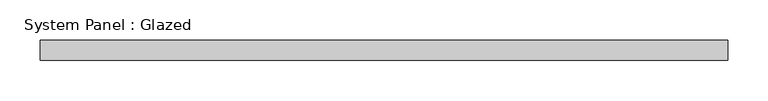
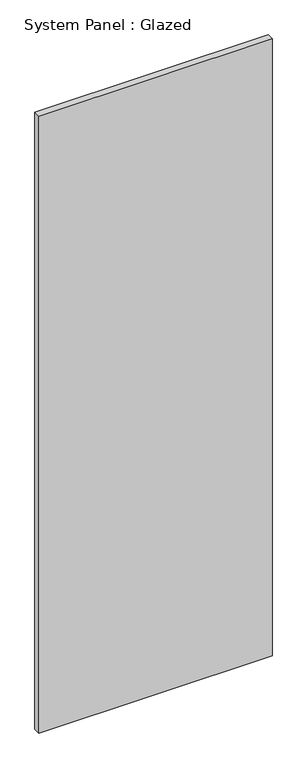
"""IFC4 building model written with IfcOpenShell, lengths in millimetres: plate geometry, System Panel : Glazed."""

from ifc_helpers import new_model, si_unit, origin, origin_with_axes, place, context, project, spatial, polyline, outline, extrude, source, transform, mapped, element, save


def system_panel_glazed_2af15f36(model_context):
    return source(origin(), model_context, "Body", "SweptSolid", [
        extrude(outline(polyline([(428.9578978, 24.5), (-428.9578978, 24.5), (-428.9578978, 49.5), (428.9578978, 49.5), (428.9578978, 24.5)])), origin_with_axes(), (0.0, 0.0, 1.0), 2400.0),
    ])


if __name__ == "__main__":
    model = new_model("IFC4")
    model_context = context("Model", 3, world=origin())
    ifc_project = project(units=[si_unit("LENGTHUNIT", "METRE", prefix="MILLI")], contexts=[model_context])
    site = spatial("IfcSite", under=ifc_project)
    building = spatial("IfcBuilding", under=site)
    placement = place(None, origin())
    system_panel_glazed_shape = system_panel_glazed_2af15f36(model_context)
    element("IfcPlate", 1, ObjectType="System Panel : Glazed", at=placement, inside=building, context=model_context, shape_type="MappedRepresentation", body=[
        mapped(system_panel_glazed_shape, transform((0.0, 0.0, 0.0), x_axis=(1.0, 0.0, 0.0), y_axis=(0.0, 1.0, 0.0), z_axis=(0.0, 0.0, 1.0))),
    ])
    save(model, "model.ifc")

# Revit data of these elements
# Type "System Panel : Glazed"
#   Keynote = "H11"
#   Construction Type Id = "GSP4R"
#   Analytic Construction = "1/8 in Pilkington single glazing"
#   Visual Light Transmittance = 0.9
#   Solar Heat Gain Coefficient = 0.86
#   Heat Transfer Coefficient (U) = 6.7069 W/(m²·K)
#   Define Thermal Properties by = 1
# Element 1 (IfcPlate, "System Panel : Glazed")
#   Materials on its faces: "Glass"
# Materials
#   "Glass": class "Glass", colour RGB 0 128 192, transparency 0.9, Description = "Soda Lime Glass", Cost = 0
